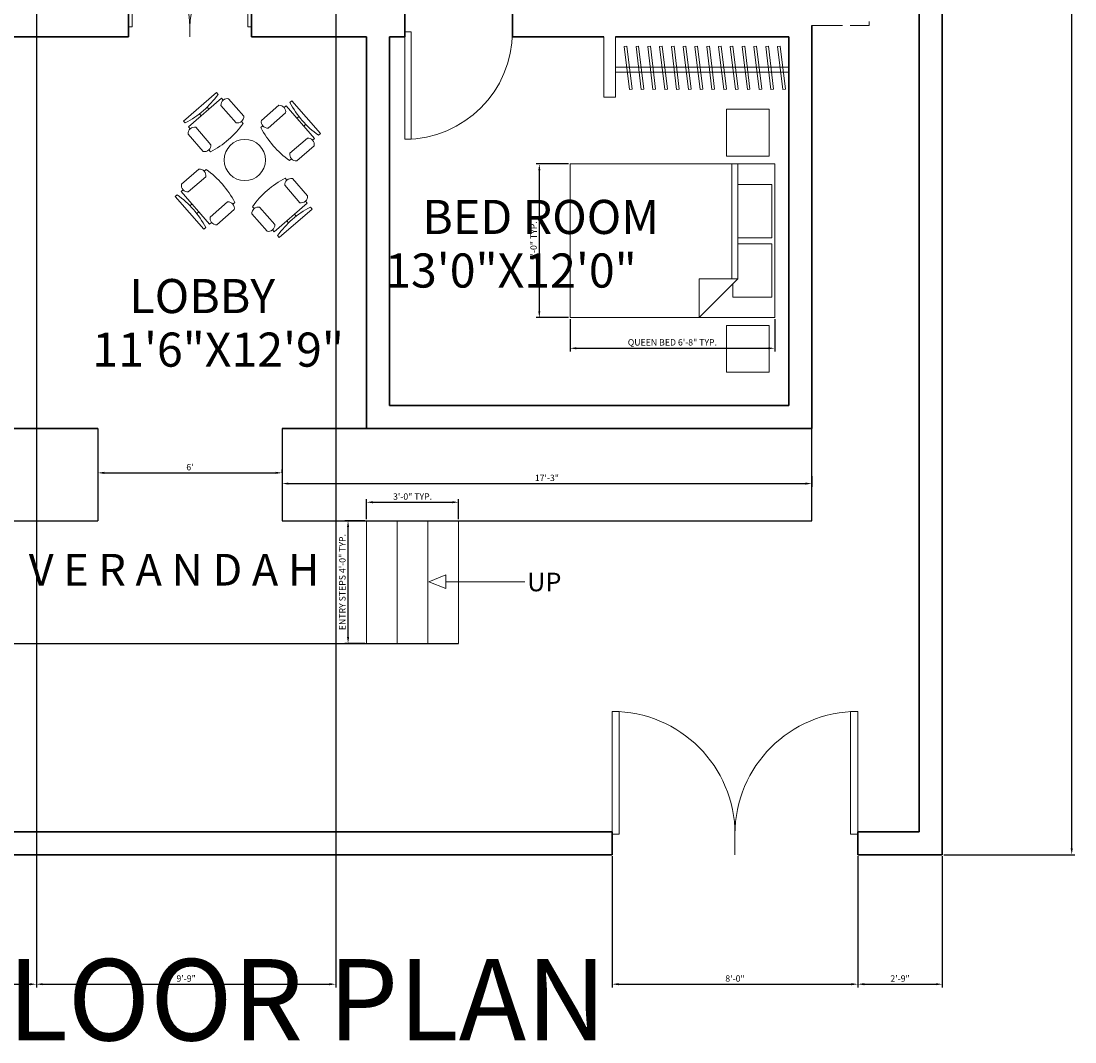
# Model space of a CAD drawing. Units: inches. Extents: x 3412 to 4225, y 13529 to 14581.
# Tile 2 of 7: x 3813 to 4225, y 13529 to 13928. Entities that reach past the tile are written whole.
import ezdxf

# ---------------------------------------------------------------- set-up
doc = ezdxf.new("R2010")
doc.units = ezdxf.units.IN
doc.linetypes.add('ACAD_ISO02W100', pattern=[15, 12, -3])
for name, color, linetype, lineweight in [('A-ANNO-DIMS', 2, 'Continuous', 13), ('A-ANNO-SYMB', 2, 'Continuous', 13), ('A-ANNO-TEXT', 7, 'Continuous', 18), ('A-ANNO-TITL', 7, 'Continuous', 35), ('A-AREA-IDEN', 7, 'Continuous', 18), ('A-DOOR', 4, 'Continuous', 18), ('A-FLOR', 7, 'Continuous', 25), ('A-FLOR-CASE', 9, 'Continuous', 18), ('A-FLOR-STRS', 3, 'Continuous', 18), ('A-FURN', 8, 'Continuous', 18), ('A-WALL', 7, 'Continuous', 35), ('A-WALL-OVHD', 8, 'ACAD_ISO02W100', 18), ('C-SITE-GATE', 4, 'Continuous', 18), ('C-SITE-WALL', 7, 'Continuous', 35)]:
    doc.layers.add(name, color=color, linetype=linetype, lineweight=lineweight)
doc.styles.get("Standard").update_dxf_attribs({"font": 'arial.ttf'})
doc.dimstyles.new('ISO-25', dxfattribs={"dimtxt": 2.5, "dimasz": 2.5, "dimexe": 1.25, "dimexo": 0.625, "dimtad": 1, "dimdec": 0, "dimlunit": 3, "dimtxsty": 'Standard', "dimcen": 2.5, "dimadec": 0, "dimazin": 0, "dimtfac": 1, "dimtdec": 0, "dimtmove": 0, "dimatfit": 3, "dimfxl": 1, "dimarcsym": 0})

# ---------------------------------------------------------------- blocks, each defined once
blk = doc.blocks.new('*U3')
for p, q in [((0, 0), (0, -5)), ((30, 0), (30, -5))]:
    blk.add_line(p, q)
blk.add_lwpolyline([(0, 0), (0, 30), (1.75, 30), (1.75, 0)], close=True)
blk.add_arc((0, 0), 30, 0, 90)
blk = doc.blocks.new('Bed - Queen')
for p, q in [((0, -80.00003), (0, 0)), ((0, 0), (59.99999, 0)), ((59.99999, 0), (59.99999, -80.00003)), ((7.99999, -1.2), (28.79998, -1.2)), ((7.99999, -14.4), (7.99999, -1.2)), ((28.79998, -1.2), (28.79998, -14.4)), ((31.19999, -1.2), (51.99999, -1.2)), ((31.19999, -14.4), (31.19999, -1.2)), ((51.99999, -1.2), (51.99999, -16.4)), ((0, -14.4), (44.8, -14.4)), ((59.99999, -29.6), (44.8, -14.4)), ((44.8, -14.4), (44.8, -29.6)), ((51.99999, -16.4), (46.79936, -16.4)), ((44.8, -16.8), (0, -16.8)), ((44.8, -29.6), (59.99999, -29.6)), ((59.99999, -80.00003), (0, -80.00003))]:
    blk.add_line(p, q)
blk = doc.blocks.new('Chair - Desk')
for p, q in [((-8.5, 0), (-8.5, -1)), ((-8.5, 0), (8.5, 0)), ((8.5, 0), (8.5, -1)), ((-8.5, -3), (-8.5, -4)), ((-8.5, -3), (8.5, -3)), ((-2, -3), (-2, -1.9355)), ((2, -1.9576), (2, -3)), ((8.5, -3), (8.5, -4)), ((-10.5, -5), (-10.5, -14)), ((-6.5, -14), (-6.5, -5)), ((6.5, -5), (6.5, -14)), ((10.5, -14), (10.5, -5)), ((-8.5, -15), (-8.5, -16)), ((8.5, -15), (8.5, -16))]:
    blk.add_line(p, q)
for centre, radius, start, end in [((-8.5, -6.5), 2.5, 36.8699, 143.1301), ((0, 34.625), 36.625, 256.5803, 283.4197), ((8.5, -6.5), 2.5, 36.8699, 143.1301), ((-8.5, -12.5), 2.5, 216.8699, 323.1301), ((0, 19.625), 36.625, 256.5803, 283.4197), ((8.5, -12.5), 2.5, 216.8699, 323.1301)]:
    blk.add_arc(centre, radius, start, end)
blk = doc.blocks.new('*U12')
blk.add_blockref('Chair - Desk', (0, 8.5))
blk = doc.blocks.new('*U13')
at = {"layer": 'A-FURN', "color": 0, "linetype": 'ByBlock', "lineweight": -2, "transparency": 16777216}
blk.add_blockref('*U12', (3901.64, 13894.79), dxfattribs=at)
for p, rotation in [((3879.85, 13874.68), 90.00000000000003), ((3921.75, 13873), 270.0000000000001), ((3899.96, 13852.89), 180)]:
    blk.add_blockref('*U12', p, dxfattribs=dict(at, rotation=rotation))
blk = doc.blocks.new('*D14')
at = {"layer": 'A-ANNO-DIMS', "color": 0, "lineweight": -2, "transparency": 16777216}
for p, q in [((3843.36, 13751.6), (3843.36, 13750.37)), ((3845.86, 13751.62), (3912.86, 13751.62)), ((3915.36, 13751.56), (3915.36, 13752.87))]:
    blk.add_line(p, q, dxfattribs=at)
at = {"layer": 'A-ANNO-DIMS', "color": 0, "transparency": 16777216}
for points in [[(3845.86, 13752.03), (3845.86, 13751.2), (3843.36, 13751.62)], [(3912.86, 13752.03), (3912.86, 13751.2), (3915.36, 13751.62)]]:
    blk.add_solid(points, dxfattribs=at)
at = {"layer": 'Defpoints', "color": 0, "transparency": 16777216}
for p in [(3843.36, 13752.22), (3915.36, 13751.62), (3915.36, 13750.93)]:
    blk.add_point(p, dxfattribs=at)
at = {"layer": 'A-ANNO-DIMS', "color": 0, "transparency": 16777216, "insert": (3879.36, 13753.52), "char_height": 2.5, "attachment_point": 5}
blk.add_mtext("6'", dxfattribs=at)
blk = doc.blocks.new('*D25')
at = {"layer": 'A-ANNO-DIMS', "color": 0, "lineweight": -2, "transparency": 16777216}
for p, q in [((3915.36, 13752.24), (3915.36, 13746.17)), ((3917.86, 13747.42), (4119.86, 13747.42)), ((4122.36, 13750.31), (4122.36, 13746.17))]:
    blk.add_line(p, q, dxfattribs=at)
at = {"layer": 'A-ANNO-DIMS', "color": 0, "transparency": 16777216}
for points in [[(3917.86, 13747.84), (3917.86, 13747.01), (3915.36, 13747.42)], [(4119.86, 13747.84), (4119.86, 13747.01), (4122.36, 13747.42)]]:
    blk.add_solid(points, dxfattribs=at)
at = {"layer": 'Defpoints', "color": 0, "transparency": 16777216}
for p in [(3915.36, 13752.87), (4122.36, 13750.93), (4122.36, 13747.42)]:
    blk.add_point(p, dxfattribs=at)
at = {"layer": 'A-ANNO-DIMS', "color": 0, "transparency": 16777216, "insert": (4018.86, 13749.33), "char_height": 2.5, "attachment_point": 5}
blk.add_mtext('17\'-3"', dxfattribs=at)
blk = doc.blocks.new('ARROW-ENTRY-STEP')
for p, q in [((30.86, 5.34), (37.49, 2.66)), ((30.86, 0), (30.86, 5.34)), ((0, 2.66), (30.86, 2.66)), ((37.49, 2.66), (30.86, 0))]:
    blk.add_line(p, q)
blk = doc.blocks.new('NIGHTSTAND')
blk.add_lwpolyline([(0, 16.62), (18.31, 16.62), (18.31, 0), (0, 0)], close=True)
blk = doc.blocks.new('WARDROBE-RAIL-ASSEMBLY')
for p, q in [((0, 0), (0, 23.57)), ((0, 23.57), (4.5, 23.57)), ((4.5, 0), (4.5, 23.57)), ((4.5, 13.79), (72.22, 13.79)), ((4.5, 11.79), (72.22, 11.79))]:
    blk.add_line(p, q)
for points in [[(9.96, 20.59), (11, 20.47), (8.96, 3.56), (7.93, 3.68)], [(14.57, 20.59), (15.61, 20.47), (13.57, 3.56), (12.54, 3.68)], [(19.18, 20.59), (20.22, 20.47), (18.18, 3.56), (17.14, 3.68)], [(23.79, 20.59), (24.82, 20.47), (22.79, 3.56), (21.75, 3.68)], [(28.4, 20.59), (29.43, 20.47), (27.4, 3.56), (26.36, 3.68)], [(33, 20.59), (34.04, 20.47), (32, 3.56), (30.97, 3.68)], [(37.61, 20.59), (38.65, 20.47), (36.61, 3.56), (35.58, 3.68)], [(42.22, 20.59), (43.26, 20.47), (41.22, 3.56), (40.18, 3.68)], [(46.83, 20.59), (47.86, 20.47), (45.83, 3.56), (44.79, 3.68)], [(51.44, 20.59), (52.47, 20.47), (50.44, 3.56), (49.4, 3.68)], [(56.05, 20.59), (57.08, 20.47), (55.04, 3.56), (54.01, 3.68)], [(60.65, 20.59), (61.69, 20.47), (59.65, 3.56), (58.62, 3.68)], [(65.26, 20.59), (66.3, 20.47), (64.26, 3.56), (63.22, 3.68)], [(69.87, 20.59), (70.91, 20.47), (68.87, 3.56), (67.83, 3.68)]]:
    blk.add_lwpolyline(points, close=True)
blk = doc.blocks.new('ENTRY-STEP-FLIGHT')
for p, q in [((0, 48), (0, 0)), ((12, 48), (12, 0)), ((24, 48), (24, 0)), ((36, 48), (36, 0))]:
    blk.add_line(p, q)
blk = doc.blocks.new('*D34')
at = {"layer": 'A-ANNO-DIMS', "color": 0, "lineweight": -2, "transparency": 16777216}
for p, q in [((4027.9, 13811.66), (4027.9, 13799.03)), ((4107.9, 13811.66), (4107.9, 13799.03)), ((4030.4, 13800.28), (4105.4, 13800.28))]:
    blk.add_line(p, q, dxfattribs=at)
at = {"layer": 'A-ANNO-DIMS', "color": 0, "transparency": 16777216}
for points in [[(4030.4, 13800.7), (4030.4, 13799.87), (4027.9, 13800.28)], [(4105.4, 13800.7), (4105.4, 13799.87), (4107.9, 13800.28)]]:
    blk.add_solid(points, dxfattribs=at)
at = {"layer": 'Defpoints', "color": 0, "transparency": 16777216}
for p in [(4027.9, 13812.28), (4107.9, 13812.28), (4107.9, 13800.28)]:
    blk.add_point(p, dxfattribs=at)
at = {"layer": 'A-ANNO-DIMS', "color": 0, "transparency": 16777216, "insert": (4067.9, 13802.28), "char_height": 2.5, "attachment_point": 5}
blk.add_mtext('QUEEN BED 6\'-8" TYP.', dxfattribs=at)
blk = doc.blocks.new('*D35')
at = {"layer": 'A-ANNO-DIMS', "color": 0, "lineweight": -2, "transparency": 16777216}
for p, q in [((4027.27, 13872.28), (4014.65, 13872.28)), ((4015.9, 13869.78), (4015.9, 13814.78)), ((4027.27, 13812.28), (4014.65, 13812.28))]:
    blk.add_line(p, q, dxfattribs=at)
at = {"layer": 'A-ANNO-DIMS', "color": 0, "transparency": 16777216}
for points in [[(4015.48, 13869.78), (4016.31, 13869.78), (4015.9, 13872.28)], [(4015.48, 13814.78), (4016.31, 13814.78), (4015.9, 13812.28)]]:
    blk.add_solid(points, dxfattribs=at)
at = {"layer": 'Defpoints', "color": 0, "transparency": 16777216}
for p in [(4027.9, 13872.28), (4015.9, 13812.28), (4027.9, 13812.28)]:
    blk.add_point(p, dxfattribs=at)
at = {"layer": 'A-ANNO-DIMS', "color": 0, "transparency": 16777216, "insert": (4014, 13842.28), "char_height": 2.5, "attachment_point": 5, "rotation": 90}
blk.add_mtext('5\'-0" TYP.', dxfattribs=at)
blk = doc.blocks.new('*D46')
at = {"layer": 'A-ANNO-DIMS', "color": 0, "lineweight": -2, "transparency": 16777216}
for p, q in [((3947.73, 13732.93), (3939.91, 13732.93)), ((3941.16, 13687.43), (3941.16, 13730.43)), ((3947.73, 13684.93), (3939.91, 13684.93))]:
    blk.add_line(p, q, dxfattribs=at)
at = {"layer": 'A-ANNO-DIMS', "color": 0, "transparency": 16777216}
for points in [[(3940.74, 13730.43), (3941.57, 13730.43), (3941.16, 13732.93)], [(3940.74, 13687.43), (3941.57, 13687.43), (3941.16, 13684.93)]]:
    blk.add_solid(points, dxfattribs=at)
at = {"layer": 'Defpoints', "color": 0, "transparency": 16777216}
for p in [(3941.16, 13732.93), (3948.36, 13732.93), (3948.36, 13684.93)]:
    blk.add_point(p, dxfattribs=at)
at = {"layer": 'A-ANNO-DIMS', "color": 0, "transparency": 16777216, "insert": (3939.24, 13708.93), "char_height": 2.5, "attachment_point": 5, "rotation": 90}
blk.add_mtext('ENTRY STEPS 4\'-0" TYP.', dxfattribs=at)
blk = doc.blocks.new('*D47')
at = {"layer": 'A-ANNO-DIMS', "color": 0, "lineweight": -2, "transparency": 16777216}
for p, q in [((3948.36, 13733.56), (3948.36, 13741.38)), ((3950.86, 13740.13), (3981.86, 13740.13)), ((3984.36, 13733.56), (3984.36, 13741.38))]:
    blk.add_line(p, q, dxfattribs=at)
at = {"layer": 'A-ANNO-DIMS', "color": 0, "transparency": 16777216}
for points in [[(3950.86, 13740.55), (3950.86, 13739.72), (3948.36, 13740.13)], [(3981.86, 13740.55), (3981.86, 13739.72), (3984.36, 13740.13)]]:
    blk.add_solid(points, dxfattribs=at)
at = {"layer": 'Defpoints', "color": 0, "transparency": 16777216}
for p in [(3984.36, 13740.13), (3948.36, 13732.93), (3984.36, 13732.93)]:
    blk.add_point(p, dxfattribs=at)
at = {"layer": 'A-ANNO-DIMS', "color": 0, "transparency": 16777216, "insert": (3966.36, 13742.03), "char_height": 2.5, "attachment_point": 5}
blk.add_mtext('3\'-0" TYP.', dxfattribs=at)
blk = doc.blocks.new('*D57')
at = {"layer": 'A-ANNO-DIMS', "color": 0, "lineweight": -2, "transparency": 16777216}
for p, q in [((4173.98, 14526.43), (4225.21, 14526.43)), ((4223.96, 13604.93), (4223.96, 14523.93)), ((4173.98, 13602.43), (4225.21, 13602.43))]:
    blk.add_line(p, q, dxfattribs=at)
at = {"layer": 'A-ANNO-DIMS', "color": 0, "transparency": 16777216}
for points in [[(4223.54, 14523.93), (4224.37, 14523.93), (4223.96, 14526.43)], [(4223.54, 13604.93), (4224.37, 13604.93), (4223.96, 13602.43)]]:
    blk.add_solid(points, dxfattribs=at)
at = {"layer": 'Defpoints', "color": 0, "transparency": 16777216}
for p in [(4173.36, 14526.43), (4223.96, 14526.43), (4173.36, 13602.43)]:
    blk.add_point(p, dxfattribs=at)
at = {"layer": 'A-ANNO-DIMS', "color": 0, "transparency": 16777216, "insert": (4222.06, 14064.43), "char_height": 2.5, "attachment_point": 5, "rotation": 90}
blk.add_mtext('77\'-0"', dxfattribs=at)
blk = doc.blocks.new('*D66')
at = {"layer": 'A-ANNO-DIMS', "color": 0, "lineweight": -2, "transparency": 16777216}
for p, q in [((3789.36, 14408.81), (3789.36, 13550.58)), ((3819.36, 14408.81), (3819.36, 13550.58)), ((3791.86, 13551.83), (3816.86, 13551.83))]:
    blk.add_line(p, q, dxfattribs=at)
at = {"layer": 'A-ANNO-DIMS', "color": 0, "transparency": 16777216}
for points in [[(3791.86, 13552.25), (3791.86, 13551.42), (3789.36, 13551.83)], [(3816.86, 13552.25), (3816.86, 13551.42), (3819.36, 13551.83)]]:
    blk.add_solid(points, dxfattribs=at)
at = {"layer": 'Defpoints', "color": 0, "transparency": 16777216}
for p in [(3789.36, 14409.43), (3819.36, 14409.43), (3819.36, 13551.83)]:
    blk.add_point(p, dxfattribs=at)
at = {"layer": 'A-ANNO-DIMS', "color": 0, "transparency": 16777216, "insert": (3804.36, 13553.73), "char_height": 2.5, "attachment_point": 5}
blk.add_mtext('2\'-6"', dxfattribs=at)
blk = doc.blocks.new('*D67')
at = {"layer": 'A-ANNO-DIMS', "color": 0, "lineweight": -2, "transparency": 16777216}
for p, q in [((3819.36, 14408.81), (3819.36, 13550.58)), ((3936.36, 14408.81), (3936.36, 13550.58)), ((3821.86, 13551.83), (3933.86, 13551.83))]:
    blk.add_line(p, q, dxfattribs=at)
at = {"layer": 'A-ANNO-DIMS', "color": 0, "transparency": 16777216}
for points in [[(3821.86, 13552.25), (3821.86, 13551.42), (3819.36, 13551.83)], [(3933.86, 13552.25), (3933.86, 13551.42), (3936.36, 13551.83)]]:
    blk.add_solid(points, dxfattribs=at)
at = {"layer": 'Defpoints', "color": 0, "transparency": 16777216}
for p in [(3819.36, 14409.43), (3936.36, 14409.43), (3936.36, 13551.83)]:
    blk.add_point(p, dxfattribs=at)
at = {"layer": 'A-ANNO-DIMS', "color": 0, "transparency": 16777216, "insert": (3877.86, 13553.73), "char_height": 2.5, "attachment_point": 5}
blk.add_mtext('9\'-9"', dxfattribs=at)
blk = doc.blocks.new('*D81')
at = {"layer": 'A-ANNO-DIMS', "color": 0, "lineweight": -2, "transparency": 16777216}
for p, q in [((4044.36, 13601.81), (4044.36, 13550.58)), ((4140.36, 13601.81), (4140.36, 13550.58)), ((4046.86, 13551.83), (4137.86, 13551.83))]:
    blk.add_line(p, q, dxfattribs=at)
at = {"layer": 'A-ANNO-DIMS', "color": 0, "transparency": 16777216}
for points in [[(4046.86, 13552.25), (4046.86, 13551.42), (4044.36, 13551.83)], [(4137.86, 13552.25), (4137.86, 13551.42), (4140.36, 13551.83)]]:
    blk.add_solid(points, dxfattribs=at)
at = {"layer": 'Defpoints', "color": 0, "transparency": 16777216}
for p in [(4044.36, 13602.43), (4140.36, 13602.43), (4140.36, 13551.83)]:
    blk.add_point(p, dxfattribs=at)
at = {"layer": 'A-ANNO-DIMS', "color": 0, "transparency": 16777216, "insert": (4092.36, 13553.73), "char_height": 2.5, "attachment_point": 5}
blk.add_mtext('8\'-0"', dxfattribs=at)
blk = doc.blocks.new('*D82')
at = {"layer": 'A-ANNO-DIMS', "color": 0, "lineweight": -2, "transparency": 16777216}
for p, q in [((4140.36, 13601.81), (4140.36, 13550.58)), ((4173.36, 13601.81), (4173.36, 13550.58)), ((4142.86, 13551.83), (4170.86, 13551.83))]:
    blk.add_line(p, q, dxfattribs=at)
at = {"layer": 'A-ANNO-DIMS', "color": 0, "transparency": 16777216}
for points in [[(4142.86, 13552.25), (4142.86, 13551.42), (4140.36, 13551.83)], [(4170.86, 13552.25), (4170.86, 13551.42), (4173.36, 13551.83)]]:
    blk.add_solid(points, dxfattribs=at)
at = {"layer": 'Defpoints', "color": 0, "transparency": 16777216}
for p in [(4140.36, 13602.43), (4173.36, 13602.43), (4173.36, 13551.83)]:
    blk.add_point(p, dxfattribs=at)
at = {"layer": 'A-ANNO-DIMS', "color": 0, "transparency": 16777216, "insert": (4156.86, 13553.73), "char_height": 2.5, "attachment_point": 5}
blk.add_mtext('2\'-9"', dxfattribs=at)

msp = doc.modelspace()

# ---------------------------------------------------------------- linework, layer by layer
at = {"layer": 'A-FLOR'}
for p, q in [((3843.36, 13768.93), (3843.36, 13732.93)), ((3915.36, 13768.93), (3915.36, 13732.93)), ((4122.36, 13732.93), (4122.36, 13768.93)), ((3624.36, 13732.93), (3843.36, 13732.93)), ((3915.36, 13732.93), (4122.36, 13732.93)), ((3774.36, 13684.93), (3984.36, 13684.93))]:
    msp.add_line(p, q, dxfattribs=at)
at = {"layer": 'A-FURN'}
msp.add_circle((3900.8, 13873.84), 8.07, dxfattribs=at)
at = {"layer": 'A-WALL'}
for p, q in [((3855.36, 13921.93), (3855.36, 13930.93)), ((3903.36, 13921.93), (3903.36, 13930.93)), ((3963.36, 13930.93), (3963.36, 13921.93)), ((4005.36, 13930.93), (4005.36, 13921.93)), ((4122.36, 13926.43), (4122.36, 13768.93)), ((3810.36, 13921.93), (3855.36, 13921.93)), ((3903.36, 13921.93), (3948.36, 13921.93)), ((3948.36, 13921.93), (3948.36, 13768.93)), ((3957.36, 13921.93), (3957.36, 13777.93)), ((3957.36, 13921.93), (3963.36, 13921.93)), ((4005.36, 13921.93), (4041.14, 13921.93)), ((4045.64, 13921.93), (4113.36, 13921.93)), ((4113.36, 13921.93), (4113.36, 13777.93)), ((3957.36, 13777.93), (4113.36, 13777.93)), ((3624.36, 13768.93), (3843.36, 13768.93)), ((3915.36, 13768.93), (4122.36, 13768.93))]:
    msp.add_line(p, q, dxfattribs=at)
at = {"layer": 'A-WALL-OVHD'}
for p in [(4144.86, 14047.93), (4122.36, 13926.43)]:
    msp.add_line(p, (4144.86, 13926.43), dxfattribs=at)
at = {"layer": 'C-SITE-WALL'}
for p, q in [((4173.36, 14526.43), (4173.36, 13602.43)), ((4164.36, 14517.43), (4164.36, 13611.43)), ((3651.36, 13611.43), (4044.36, 13611.43)), ((4044.36, 13611.43), (4044.36, 13602.43)), ((4140.36, 13611.43), (4140.36, 13602.43)), ((4140.36, 13611.43), (4164.36, 13611.43)), ((3651.36, 13602.43), (4044.36, 13602.43)), ((4140.36, 13602.43), (4173.36, 13602.43))]:
    msp.add_line(p, q, dxfattribs=at)

# ---------------------------------------------------------------- block references
at = {"layer": 'A-ANNO-SYMB', "extrusion": (0, 0, -1), "zscale": -1}
msp.add_blockref('ARROW-ENTRY-STEP', (-4010.25, 13706.43), dxfattribs=at)
at = {"layer": 'A-DOOR', "yscale": 0.8, "zscale": 0.8}
for p, xscale in [((3855.36, 13925.93), 0.8), ((3903.36, 13925.93), -0.8)]:
    msp.add_blockref('*U3', p, dxfattribs=dict(at, xscale=xscale))
at = {"layer": 'A-DOOR', "xscale": -1.399999999999999, "yscale": 1.399999999999999, "zscale": 1.399999999999999, "rotation": 180}
msp.add_blockref('*U3', (3963.36, 13923.93), dxfattribs=at)
at = {"layer": 'A-FLOR-CASE', "extrusion": (0, 0, -1), "zscale": -1, "rotation": 180}
msp.add_blockref('WARDROBE-RAIL-ASSEMBLY', (-4041.14, 13921.93), dxfattribs=at)
at = {"layer": 'A-FLOR-STRS'}
msp.add_blockref('ENTRY-STEP-FLIGHT', (3948.36, 13684.93), dxfattribs=at)
at = {"layer": 'A-FURN'}
for name, p, rotation in [('*U13', (10065.99, 844.81), 41.02602795982508), ('NIGHTSTAND', (4089.1, 13893.64), 270.00000000001), ('Bed - Queen', (4107.9, 13872.28), 270)]:
    msp.add_blockref(name, p, dxfattribs=dict(at, rotation=rotation))
at = {"layer": 'A-FURN', "extrusion": (0, 0, -1), "zscale": -1, "rotation": 90.00000000000531}
msp.add_blockref('NIGHTSTAND', (-4089.1, 13790.92), dxfattribs=at)
at = {"layer": 'C-SITE-GATE', "yscale": 1.599999999999999, "zscale": 1.599999999999999}
for p, xscale in [((4044.36, 13610.43), 1.599999999999999), ((4140.36, 13610.43), -1.599999999999999)]:
    msp.add_blockref('*U3', p, dxfattribs=dict(at, xscale=xscale))

# ---------------------------------------------------------------- texts
at = {"layer": 'A-ANNO-TEXT'}
msp.add_text('UP', height=7.282, dxfattribs=at).set_placement((4011.1, 13705.34))
at = {"layer": 'A-ANNO-TITL'}
msp.add_text('GROUND FLOOR PLAN', height=31.8222, dxfattribs=at).set_placement((3592.1, 13529.85))
at = {"layer": 'A-AREA-IDEN'}
for s, height, p in [('BED ROOM', 13.329, (3970.15, 13844.93)), ('13\'0"X12\'0"', 13.3293, (3955.65, 13824)), ('LOBBY', 13.329, (3855.71, 13814.02)), ('11\'6"X12\'9"', 13.3293, (3841.21, 13793.09)), ('V E R A N D A H', 12.3861, (3816.36, 13707.57))]:
    msp.add_text(s, height=height, dxfattribs=at).set_placement(p)

# ---------------------------------------------------------------- dimensions: what is measured, and where the dimension line sits
at = {"layer": 'A-ANNO-DIMS'}
dim = msp.add_linear_dim(base=(4223.96, 14526.43), p1=(4173.36, 13602.43), p2=(4173.36, 14526.43), angle=90, dimstyle='ISO-25', override={"dimdec": 1, "dimlfac": 1, "dimrnd": 0, "dimzin": 1, "dimdsep": 46, "dimlunit": 4, "dimfrac": 2}, dxfattribs=at)
dim.commit()
dim.dimension.update_dxf_attribs({"geometry": '*D57', "text_midpoint": (4222.06, 14064.43)})
for base, p1, p2, override, picture, middle in [((3819.36, 13551.83), (3789.36, 14409.43), (3819.36, 14409.43), {"dimdec": 1, "dimlfac": 1, "dimrnd": 0, "dimzin": 1, "dimdsep": 46, "dimlunit": 4, "dimfrac": 2}, '*D66', (3804.36, 13553.73)), ((3936.36, 13551.83), (3819.36, 14409.43), (3936.36, 14409.43), {"dimdec": 1, "dimlfac": 1, "dimrnd": 0, "dimzin": 1, "dimdsep": 46, "dimlunit": 4, "dimfrac": 2}, '*D67', (3877.86, 13553.73)), ((3915.36, 13751.62), (3843.36, 13752.22), (3915.36, 13750.93), {"dimclrd": 0, "dimclre": 0, "dimclrt": 0}, '*D14', (3879.36, 13753.52)), ((4122.36, 13747.42), (3915.36, 13752.87), (4122.36, 13750.93), {"dimclrd": 0, "dimclre": 0, "dimclrt": 0}, '*D25', (4018.86, 13749.33)), ((4140.36, 13551.83), (4044.36, 13602.43), (4140.36, 13602.43), {"dimdec": 1, "dimlfac": 1, "dimrnd": 0, "dimzin": 1, "dimdsep": 46, "dimlunit": 4, "dimfrac": 2}, '*D81', (4092.36, 13553.73)), ((4173.36, 13551.83), (4140.36, 13602.43), (4173.36, 13602.43), {"dimdec": 1, "dimlfac": 1, "dimrnd": 0, "dimzin": 1, "dimdsep": 46, "dimlunit": 4, "dimfrac": 2}, '*D82', (4156.86, 13553.73))]:
    dim = msp.add_linear_dim(base=base, p1=p1, p2=p2, dimstyle='ISO-25', override=override, dxfattribs=at)
    dim.commit()
    dim.dimension.update_dxf_attribs({"geometry": picture, "text_midpoint": middle})
for base, p1, p2, angle, text, picture, middle in [((4015.9, 13812.28), (4027.9, 13872.28), (4027.9, 13812.28), 270, '<> TYP.', '*D35', (4014, 13842.28)), ((3941.16, 13732.93), (3948.36, 13684.93), (3948.36, 13732.93), 90, 'ENTRY STEPS <> TYP.', '*D46', (3939.24, 13708.93))]:
    dim = msp.add_linear_dim(base=base, p1=p1, p2=p2, angle=angle, text=text, dimstyle='ISO-25', override={"dimdec": 1, "dimlfac": 1, "dimrnd": 0, "dimzin": 1, "dimdsep": 46, "dimlunit": 4, "dimfrac": 2}, dxfattribs=at)
    dim.commit()
    dim.dimension.update_dxf_attribs({"geometry": picture, "text_midpoint": middle})
for base, p1, p2, text, picture, middle in [((4107.9, 13800.28), (4027.9, 13812.28), (4107.9, 13812.28), 'QUEEN BED <> TYP.', '*D34', (4067.9, 13802.28)), ((3984.36, 13740.13), (3948.36, 13732.93), (3984.36, 13732.93), '<> TYP.', '*D47', (3966.36, 13742.03))]:
    dim = msp.add_linear_dim(base=base, p1=p1, p2=p2, text=text, dimstyle='ISO-25', override={"dimdec": 1, "dimlfac": 1, "dimrnd": 0, "dimzin": 1, "dimdsep": 46, "dimlunit": 4, "dimfrac": 2}, dxfattribs=at)
    dim.commit()
    dim.dimension.update_dxf_attribs({"geometry": picture, "text_midpoint": middle})

doc.saveas('drawing.dxf')
